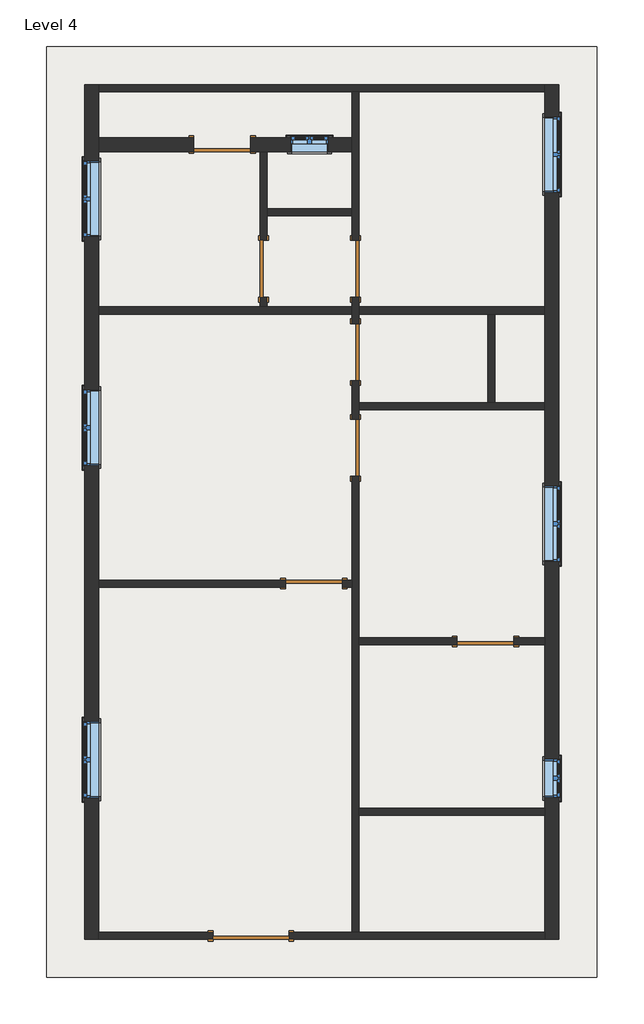
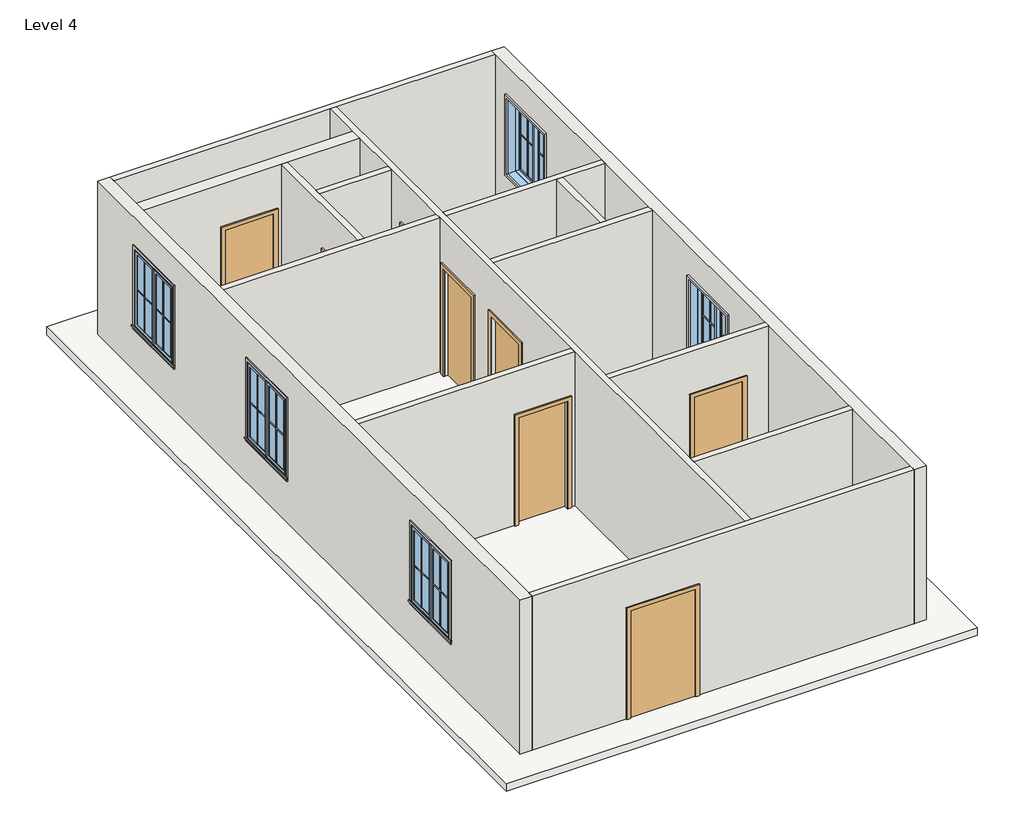
# One storey, incomplete: 28 proxies, 15 walls, 8 doors, 7 windows, 1 slab.
"""IFC4 building model written with IfcOpenShell, lengths in millimetres."""

from ifc_helpers import new_model, si_unit, frame, origin, place, context, project, spatial, polyline, outline, extrude, faceted_brep, transform, mapped, element, save
from components import muntin_pattern_2x2_muntin_pattern_2x2_6dad3731, muntin_pattern_2x2_muntin_pattern_2x2_a30a3345, muntin_pattern_2x2_muntin_pattern_2x2_53152e2c, muntin_pattern_2x2_muntin_pattern_2x2_e8f3e573, trim_window_exterior_flat_with_sill_92b9b949, trim_window_exterior_flat_with_sill_a665a915, trim_window_interior_flat_picture_frame_3bb882cf, trim_window_interior_flat_picture_frame_d485c387, door_a90ba1ad, door_e5f9f3c4, door_305aa2a5, door_6ea84ebe, window_c417fced, window_8377141f

model = new_model("IFC4")

# Units and contexts
model_context = context("Model", 3, world=origin())
ifc_project = project(units=[si_unit("LENGTHUNIT", "METRE", prefix="MILLI")], contexts=[model_context])

# Site, building, storey
site = spatial("IfcSite", under=ifc_project)
building = spatial("IfcBuilding", under=site)
storey = spatial("IfcBuildingStorey", under=building, Name="Level 4", Elevation=9144.0)

# Proxies
placement = place(None, origin())
muntin_pattern_2x2_muntin_pattern_2x2_shape = muntin_pattern_2x2_muntin_pattern_2x2_6dad3731(model_context)
element("IfcBuildingElementProxy", 1, Name="Muntin Pattern_2x2 : Muntin Pattern_2x2", ObjectType="Muntin Pattern_2x2 : Muntin Pattern_2x2", at=placement, inside=storey, context=model_context, shape_type="MappedRepresentation", body=[
    mapped(muntin_pattern_2x2_muntin_pattern_2x2_shape, transform((1279.525, 8669.3375, 10128.25), x_axis=(0.0, 1.0, 0.0), y_axis=(-1.0, 0.0, 0.0), z_axis=(0.0, 0.0, 1.0))),
])
element("IfcBuildingElementProxy", 2, Name="Muntin Pattern_2x2 : Muntin Pattern_2x2", ObjectType="Muntin Pattern_2x2 : Muntin Pattern_2x2", at=placement, inside=storey, context=model_context, shape_type="MappedRepresentation", body=[
    mapped(muntin_pattern_2x2_muntin_pattern_2x2_shape, transform((1279.525, 3341.6875, 10128.25), x_axis=(0.0, 1.0, 0.0), y_axis=(-1.0, 0.0, 0.0), z_axis=(0.0, 0.0, 1.0))),
])
element("IfcBuildingElementProxy", 3, Name="Muntin Pattern_2x2 : Muntin Pattern_2x2", ObjectType="Muntin Pattern_2x2 : Muntin Pattern_2x2", at=placement, inside=storey, context=model_context, shape_type="MappedRepresentation", body=[
    mapped(muntin_pattern_2x2_muntin_pattern_2x2_shape, transform((8880.475, 7732.7125, 10128.25), x_axis=(0.0, -1.0, 0.0), y_axis=(1.0, 0.0, 0.0), z_axis=(0.0, 0.0, 1.0))),
])
element("IfcBuildingElementProxy", 4, Name="Muntin Pattern_2x2 : Muntin Pattern_2x2", ObjectType="Muntin Pattern_2x2 : Muntin Pattern_2x2", at=placement, inside=storey, context=model_context, shape_type="MappedRepresentation", body=[
    mapped(muntin_pattern_2x2_muntin_pattern_2x2_shape, transform((8880.475, 13657.2625, 10128.25), x_axis=(0.0, -1.0, 0.0), y_axis=(1.0, 0.0, 0.0), z_axis=(0.0, 0.0, 1.0))),
])
element("IfcBuildingElementProxy", 5, Name="Muntin Pattern_2x2 : Muntin Pattern_2x2", ObjectType="Muntin Pattern_2x2 : Muntin Pattern_2x2", at=placement, inside=storey, context=model_context, shape_type="MappedRepresentation", body=[
    mapped(muntin_pattern_2x2_muntin_pattern_2x2_shape, transform((1279.525, 12339.6375, 10128.25), x_axis=(0.0, 1.0, 0.0), y_axis=(-1.0, 0.0, 0.0), z_axis=(0.0, 0.0, 1.0))),
])
muntin_pattern_2x2_muntin_pattern_2x2_2_shape = muntin_pattern_2x2_muntin_pattern_2x2_a30a3345(model_context)
element("IfcBuildingElementProxy", 6, Name="Muntin Pattern_2x2 : Muntin Pattern_2x2", ObjectType="Muntin Pattern_2x2 : Muntin Pattern_2x2", at=placement, inside=storey, context=model_context, shape_type="MappedRepresentation", body=[
    mapped(muntin_pattern_2x2_muntin_pattern_2x2_2_shape, transform((1279.525, 9275.7625, 10128.25), x_axis=(0.0, -1.0, 0.0), y_axis=(1.0, 0.0, 0.0), z_axis=(0.0, 0.0, 1.0))),
])
element("IfcBuildingElementProxy", 7, Name="Muntin Pattern_2x2 : Muntin Pattern_2x2", ObjectType="Muntin Pattern_2x2 : Muntin Pattern_2x2", at=placement, inside=storey, context=model_context, shape_type="MappedRepresentation", body=[
    mapped(muntin_pattern_2x2_muntin_pattern_2x2_2_shape, transform((1279.525, 3948.1125, 10128.25), x_axis=(0.0, -1.0, 0.0), y_axis=(1.0, 0.0, 0.0), z_axis=(0.0, 0.0, 1.0))),
])
element("IfcBuildingElementProxy", 8, Name="Muntin Pattern_2x2 : Muntin Pattern_2x2", ObjectType="Muntin Pattern_2x2 : Muntin Pattern_2x2", at=placement, inside=storey, context=model_context, shape_type="MappedRepresentation", body=[
    mapped(muntin_pattern_2x2_muntin_pattern_2x2_2_shape, transform((8880.475, 7126.2875, 10128.25), x_axis=(0.0, 1.0, 0.0), y_axis=(-1.0, 0.0, 0.0), z_axis=(0.0, 0.0, 1.0))),
])
element("IfcBuildingElementProxy", 9, Name="Muntin Pattern_2x2 : Muntin Pattern_2x2", ObjectType="Muntin Pattern_2x2 : Muntin Pattern_2x2", at=placement, inside=storey, context=model_context, shape_type="MappedRepresentation", body=[
    mapped(muntin_pattern_2x2_muntin_pattern_2x2_2_shape, transform((8880.475, 13050.8375, 10128.25), x_axis=(0.0, 1.0, 0.0), y_axis=(-1.0, 0.0, 0.0), z_axis=(0.0, 0.0, 1.0))),
])
element("IfcBuildingElementProxy", 10, Name="Muntin Pattern_2x2 : Muntin Pattern_2x2", ObjectType="Muntin Pattern_2x2 : Muntin Pattern_2x2", at=placement, inside=storey, context=model_context, shape_type="MappedRepresentation", body=[
    mapped(muntin_pattern_2x2_muntin_pattern_2x2_2_shape, transform((1279.525, 12946.0625, 10128.25), x_axis=(0.0, -1.0, 0.0), y_axis=(1.0, 0.0, 0.0), z_axis=(0.0, 0.0, 1.0))),
])
muntin_pattern_2x2_muntin_pattern_2x2_3_shape = muntin_pattern_2x2_muntin_pattern_2x2_53152e2c(model_context)
element("IfcBuildingElementProxy", 11, Name="Muntin Pattern_2x2 : Muntin Pattern_2x2", ObjectType="Muntin Pattern_2x2 : Muntin Pattern_2x2", at=placement, inside=storey, context=model_context, shape_type="MappedRepresentation", body=[
    mapped(muntin_pattern_2x2_muntin_pattern_2x2_3_shape, transform((4732.3375, 13617.575, 10128.25), x_axis=(1.0, 0.0, 0.0), y_axis=(0.0, 1.0, 0.0), z_axis=(0.0, 0.0, 1.0))),
])
element("IfcBuildingElementProxy", 12, Name="Muntin Pattern_2x2 : Muntin Pattern_2x2", ObjectType="Muntin Pattern_2x2 : Muntin Pattern_2x2", at=placement, inside=storey, context=model_context, shape_type="MappedRepresentation", body=[
    mapped(muntin_pattern_2x2_muntin_pattern_2x2_3_shape, transform((8880.475, 3497.2625, 10128.25), x_axis=(0.0, -1.0, 0.0), y_axis=(1.0, 0.0, 0.0), z_axis=(0.0, 0.0, 1.0))),
])
muntin_pattern_2x2_muntin_pattern_2x2_4_shape = muntin_pattern_2x2_muntin_pattern_2x2_e8f3e573(model_context)
element("IfcBuildingElementProxy", 13, Name="Muntin Pattern_2x2 : Muntin Pattern_2x2", ObjectType="Muntin Pattern_2x2 : Muntin Pattern_2x2", at=placement, inside=storey, context=model_context, shape_type="MappedRepresentation", body=[
    mapped(muntin_pattern_2x2_muntin_pattern_2x2_4_shape, transform((5033.9625, 13617.575, 10128.25), x_axis=(-1.0, 0.0, 0.0), y_axis=(0.0, -1.0, 0.0), z_axis=(0.0, 0.0, 1.0))),
])
element("IfcBuildingElementProxy", 14, Name="Muntin Pattern_2x2 : Muntin Pattern_2x2", ObjectType="Muntin Pattern_2x2 : Muntin Pattern_2x2", at=placement, inside=storey, context=model_context, shape_type="MappedRepresentation", body=[
    mapped(muntin_pattern_2x2_muntin_pattern_2x2_4_shape, transform((8880.475, 3195.6375, 10128.25), x_axis=(0.0, 1.0, 0.0), y_axis=(-1.0, 0.0, 0.0), z_axis=(0.0, 0.0, 1.0))),
])
trim_window_exterior_flat_with_sill_shape = trim_window_exterior_flat_with_sill_92b9b949(model_context)
element("IfcBuildingElementProxy", 15, Name="Trim-Window-Exterior-Flat : with Sill", ObjectType="Trim-Window-Exterior-Flat : with Sill", at=placement, inside=storey, context=model_context, shape_type="MappedRepresentation", body=[
    mapped(trim_window_exterior_flat_with_sill_shape, transform((1270.0, 8972.55, 11582.4), x_axis=(0.0, -1.0, 0.0), y_axis=(0.0, 0.0, 1.0), z_axis=(-1.0, 0.0, 0.0))),
])
element("IfcBuildingElementProxy", 16, Name="Trim-Window-Exterior-Flat : with Sill", ObjectType="Trim-Window-Exterior-Flat : with Sill", at=placement, inside=storey, context=model_context, shape_type="MappedRepresentation", body=[
    mapped(trim_window_exterior_flat_with_sill_shape, transform((1270.0, 3644.9, 11582.4), x_axis=(0.0, -1.0, 0.0), y_axis=(0.0, 0.0, 1.0), z_axis=(-1.0, 0.0, 0.0))),
])
element("IfcBuildingElementProxy", 17, Name="Trim-Window-Exterior-Flat : with Sill", ObjectType="Trim-Window-Exterior-Flat : with Sill", at=placement, inside=storey, context=model_context, shape_type="MappedRepresentation", body=[
    mapped(trim_window_exterior_flat_with_sill_shape, transform((8890.0, 7429.5, 11582.4), x_axis=(0.0, 1.0, 0.0), y_axis=(0.0, 0.0, 1.0), z_axis=(1.0, 0.0, 0.0))),
])
element("IfcBuildingElementProxy", 18, Name="Trim-Window-Exterior-Flat : with Sill", ObjectType="Trim-Window-Exterior-Flat : with Sill", at=placement, inside=storey, context=model_context, shape_type="MappedRepresentation", body=[
    mapped(trim_window_exterior_flat_with_sill_shape, transform((8890.0, 13354.05, 11582.4), x_axis=(0.0, 1.0, 0.0), y_axis=(0.0, 0.0, 1.0), z_axis=(1.0, 0.0, 0.0))),
])
element("IfcBuildingElementProxy", 19, Name="Trim-Window-Exterior-Flat : with Sill", ObjectType="Trim-Window-Exterior-Flat : with Sill", at=placement, inside=storey, context=model_context, shape_type="MappedRepresentation", body=[
    mapped(trim_window_exterior_flat_with_sill_shape, transform((1270.0, 12642.85, 11582.4), x_axis=(0.0, -1.0, 0.0), y_axis=(0.0, 0.0, 1.0), z_axis=(-1.0, 0.0, 0.0))),
])
trim_window_exterior_flat_with_sill_2_shape = trim_window_exterior_flat_with_sill_a665a915(model_context)
element("IfcBuildingElementProxy", 20, Name="Trim-Window-Exterior-Flat : with Sill", ObjectType="Trim-Window-Exterior-Flat : with Sill", at=placement, inside=storey, context=model_context, shape_type="MappedRepresentation", body=[
    mapped(trim_window_exterior_flat_with_sill_2_shape, transform((4883.15, 13627.1, 10972.8), x_axis=(-1.0, 0.0, 0.0), y_axis=(0.0, 0.0, 1.0), z_axis=(0.0, 1.0, 0.0))),
])
element("IfcBuildingElementProxy", 21, Name="Trim-Window-Exterior-Flat : with Sill", ObjectType="Trim-Window-Exterior-Flat : with Sill", at=placement, inside=storey, context=model_context, shape_type="MappedRepresentation", body=[
    mapped(trim_window_exterior_flat_with_sill_2_shape, transform((8890.0, 3346.45, 10972.8), x_axis=(0.0, 1.0, 0.0), y_axis=(0.0, 0.0, 1.0), z_axis=(1.0, 0.0, 0.0))),
])
trim_window_interior_flat_picture_frame_shape = trim_window_interior_flat_picture_frame_3bb882cf(model_context)
element("IfcBuildingElementProxy", 22, Name="Trim-Window-Interior-Flat : Picture Frame", ObjectType="Trim-Window-Interior-Flat : Picture Frame", at=placement, inside=storey, context=model_context, shape_type="MappedRepresentation", body=[
    mapped(trim_window_interior_flat_picture_frame_shape, transform((1498.6, 8972.55, 11582.4), x_axis=(0.0, 1.0, 0.0), y_axis=(0.0, 0.0, 1.0), z_axis=(1.0, 0.0, 0.0))),
])
element("IfcBuildingElementProxy", 23, Name="Trim-Window-Interior-Flat : Picture Frame", ObjectType="Trim-Window-Interior-Flat : Picture Frame", at=placement, inside=storey, context=model_context, shape_type="MappedRepresentation", body=[
    mapped(trim_window_interior_flat_picture_frame_shape, transform((1498.6, 3644.9, 11582.4), x_axis=(0.0, 1.0, 0.0), y_axis=(0.0, 0.0, 1.0), z_axis=(1.0, 0.0, 0.0))),
])
element("IfcBuildingElementProxy", 24, Name="Trim-Window-Interior-Flat : Picture Frame", ObjectType="Trim-Window-Interior-Flat : Picture Frame", at=placement, inside=storey, context=model_context, shape_type="MappedRepresentation", body=[
    mapped(trim_window_interior_flat_picture_frame_shape, transform((8661.4, 7429.5, 11582.4), x_axis=(0.0, -1.0, 0.0), y_axis=(0.0, 0.0, 1.0), z_axis=(-1.0, 0.0, 0.0))),
])
element("IfcBuildingElementProxy", 25, Name="Trim-Window-Interior-Flat : Picture Frame", ObjectType="Trim-Window-Interior-Flat : Picture Frame", at=placement, inside=storey, context=model_context, shape_type="MappedRepresentation", body=[
    mapped(trim_window_interior_flat_picture_frame_shape, transform((8661.4, 13354.05, 11582.4), x_axis=(0.0, -1.0, 0.0), y_axis=(0.0, 0.0, 1.0), z_axis=(-1.0, 0.0, 0.0))),
])
element("IfcBuildingElementProxy", 26, Name="Trim-Window-Interior-Flat : Picture Frame", ObjectType="Trim-Window-Interior-Flat : Picture Frame", at=placement, inside=storey, context=model_context, shape_type="MappedRepresentation", body=[
    mapped(trim_window_interior_flat_picture_frame_shape, transform((1498.6, 12642.85, 11582.4), x_axis=(0.0, 1.0, 0.0), y_axis=(0.0, 0.0, 1.0), z_axis=(1.0, 0.0, 0.0))),
])
trim_window_interior_flat_picture_frame_2_shape = trim_window_interior_flat_picture_frame_d485c387(model_context)
element("IfcBuildingElementProxy", 27, Name="Trim-Window-Interior-Flat : Picture Frame", ObjectType="Trim-Window-Interior-Flat : Picture Frame", at=placement, inside=storey, context=model_context, shape_type="MappedRepresentation", body=[
    mapped(trim_window_interior_flat_picture_frame_2_shape, transform((4883.15, 13398.5, 10972.8), x_axis=(1.0, 0.0, 0.0), y_axis=(0.0, 0.0, 1.0), z_axis=(0.0, -1.0, 0.0))),
])
element("IfcBuildingElementProxy", 28, Name="Trim-Window-Interior-Flat : Picture Frame", ObjectType="Trim-Window-Interior-Flat : Picture Frame", at=placement, inside=storey, context=model_context, shape_type="MappedRepresentation", body=[
    mapped(trim_window_interior_flat_picture_frame_2_shape, transform((8661.4, 3346.45, 10972.8), x_axis=(0.0, -1.0, 0.0), y_axis=(0.0, 0.0, 1.0), z_axis=(-1.0, 0.0, 0.0))),
])

# Doors
door_shape = door_a90ba1ad(model_context)
element("IfcDoor", 29, ObjectType="Single-Flush : 36\" x 84\"", at=placement, inside=storey, context=model_context, shape_type="MappedRepresentation", body=[
    mapped(door_shape, transform((3479.8, 13512.8, 9144.0), x_axis=(1.0, 0.0, 0.0), y_axis=(0.0, 1.0, 0.0), z_axis=(0.0, 0.0, 1.0))),
])
door_2_shape = door_e5f9f3c4(model_context)
element("IfcDoor", 30, ObjectType="Single-Flush : 36\" x 84\"", at=placement, inside=storey, context=model_context, shape_type="MappedRepresentation", body=[
    mapped(door_2_shape, transform((5619.75, 11518.9, 9144.0), x_axis=(0.0, -1.0, 0.0), y_axis=(1.0, 0.0, 0.0), z_axis=(0.0, 0.0, 1.0))),
])
element("IfcDoor", 31, ObjectType="Single-Flush : 36\" x 84\"", at=placement, inside=storey, context=model_context, shape_type="MappedRepresentation", body=[
    mapped(door_2_shape, transform((4953.0, 6470.65, 9144.0), x_axis=(1.0, 0.0, 0.0), y_axis=(0.0, 1.0, 0.0), z_axis=(0.0, 0.0, 1.0))),
])
element("IfcDoor", 32, ObjectType="Single-Flush : 36\" x 84\"", at=placement, inside=storey, context=model_context, shape_type="MappedRepresentation", body=[
    mapped(door_2_shape, transform((7708.9, 5543.55, 9144.0), x_axis=(-1.0, 0.0, 0.0), y_axis=(0.0, -1.0, 0.0), z_axis=(0.0, 0.0, 1.0))),
])
door_3_shape = door_305aa2a5(model_context)
element("IfcDoor", 33, ObjectType="Single-Flush : 36\" x 84\"", at=placement, inside=storey, context=model_context, shape_type="MappedRepresentation", body=[
    mapped(door_3_shape, transform((4146.55, 11518.9, 9144.0), x_axis=(0.0, -1.0, 0.0), y_axis=(1.0, 0.0, 0.0), z_axis=(0.0, 0.0, 1.0))),
])
element("IfcDoor", 34, ObjectType="Single-Flush : 36\" x 84\"", at=placement, inside=storey, context=model_context, shape_type="MappedRepresentation", body=[
    mapped(door_3_shape, transform((5619.75, 10185.4, 9144.0), x_axis=(0.0, 1.0, 0.0), y_axis=(-1.0, 0.0, 0.0), z_axis=(0.0, 0.0, 1.0))),
])
element("IfcDoor", 35, ObjectType="Single-Flush : 36\" x 84\"", at=placement, inside=storey, context=model_context, shape_type="MappedRepresentation", body=[
    mapped(door_3_shape, transform((5619.75, 8648.7, 9144.0), x_axis=(0.0, 1.0, 0.0), y_axis=(-1.0, 0.0, 0.0), z_axis=(0.0, 0.0, 1.0))),
])
door_4_shape = door_6ea84ebe(model_context)
element("IfcDoor", 36, ObjectType="Single-Flush : 48\" x 84\"", at=placement, inside=storey, context=model_context, shape_type="MappedRepresentation", body=[
    mapped(door_4_shape, transform((3943.35, 819.15, 9144.0), x_axis=(-1.0, 0.0, 0.0), y_axis=(0.0, -1.0, 0.0), z_axis=(0.0, 0.0, 1.0))),
])

# Slab
element("IfcSlab", 37, ObjectType="Generic - 12\"", at=placement, inside=storey, context=model_context, shape_type="SweptSolid", body=[
    extrude(outline(polyline([(9499.6, 15087.6), (9499.6, 152.4), (660.4, 152.4), (660.4, 15087.6), (9499.6, 15087.6)])), frame((0.0, 0.0, 8991.6), z_axis=(0.0, 0.0, 1.0), x_axis=(1.0, 0.0, 0.0)), (0.0, 0.0, 1.0), 152.4),
])

# Walls
element("IfcWall", 38, ObjectType="Generic - 5\"", at=placement, inside=storey, context=model_context, shape_type="Brep", body=[
    faceted_brep([(1498.6, 14363.7, 9144.0), (5562.6, 14363.7, 9144.0), (5676.9, 14363.7, 9144.0), (8661.4, 14363.7, 9144.0), (8661.4, 14363.7, 12192.0), (5676.9, 14363.7, 12192.0), (5562.6, 14363.7, 12192.0), (1498.6, 14363.7, 12192.0), (1498.6, 14478.0, 9144.0), (1498.6, 14478.0, 12192.0), (8661.4, 14478.0, 12192.0), (8661.4, 14478.0, 9144.0)], [[[0, 1, 2, 3, 4, 5, 6, 7]], [[8, 9, 10, 11]], [[3, 2, 1, 0, 8, 11]], [[7, 6, 5, 4, 10, 9]], [[4, 3, 11, 10]], [[0, 7, 9, 8]]]),
])
element("IfcWall", 39, ObjectType="Generic - 5\"", at=placement, inside=storey, context=model_context, shape_type="Brep", body=[
    faceted_brep([(1498.6, 762.0, 9144.0), (3333.75, 762.0, 9144.0), (3333.75, 762.0, 11277.6), (4552.95, 762.0, 11277.6), (4552.95, 762.0, 9144.0), (8661.4, 762.0, 9144.0), (8661.4, 762.0, 12192.0), (1498.6, 762.0, 12192.0), (3333.75, 876.3, 11277.6), (3333.75, 876.3, 9144.0), (1498.6, 876.3, 9144.0), (1498.6, 876.3, 12192.0), (5562.6, 876.3, 12192.0), (5676.9, 876.3, 12192.0), (8661.4, 876.3, 12192.0), (8661.4, 876.3, 9144.0), (5676.9, 876.3, 9144.0), (5562.6, 876.3, 9144.0), (4552.95, 876.3, 9144.0), (4552.95, 876.3, 11277.6)], [[[0, 1, 2, 3, 4, 5, 6, 7]], [[8, 9, 10, 11, 12, 13, 14, 15, 16, 17, 18, 19]], [[10, 9, 1, 0]], [[18, 17, 16, 15, 5, 4]], [[7, 6, 14, 13, 12, 11]], [[6, 5, 15, 14]], [[0, 7, 11, 10]], [[2, 1, 9, 8]], [[3, 2, 8, 19]], [[4, 3, 19, 18]]]),
])
element("IfcWall", 40, ObjectType="Generic - 5\"", at=placement, inside=storey, context=model_context, shape_type="Brep", body=[
    faceted_brep([(5562.6, 9728.2, 9144.0), (5562.6, 9105.9, 9144.0), (5562.6, 9105.9, 11277.6), (5562.6, 8191.5, 11277.6), (5562.6, 8191.5, 9144.0), (5562.6, 6527.8, 9144.0), (5562.6, 6413.5, 9144.0), (5562.6, 876.3, 9144.0), (5562.6, 876.3, 12192.0), (5562.6, 6413.5, 12192.0), (5562.6, 6527.8, 12192.0), (5562.6, 10795.0, 12192.0), (5562.6, 10909.3, 12192.0), (5562.6, 12369.8, 12192.0), (5562.6, 12484.1, 12192.0), (5562.6, 13398.5, 12192.0), (5562.6, 13627.1, 12192.0), (5562.6, 14363.7, 12192.0), (5562.6, 14363.7, 9144.0), (5562.6, 13627.1, 9144.0), (5562.6, 13398.5, 9144.0), (5562.6, 12484.1, 9144.0), (5562.6, 12369.8, 9144.0), (5562.6, 11976.1, 9144.0), (5562.6, 11976.1, 11277.6), (5562.6, 11061.7, 11277.6), (5562.6, 11061.7, 9144.0), (5562.6, 10909.3, 9144.0), (5562.6, 10795.0, 9144.0), (5562.6, 10642.6, 9144.0), (5562.6, 10642.6, 11277.6), (5562.6, 9728.2, 11277.6), (5676.9, 9105.9, 11277.6), (5676.9, 9105.9, 9144.0), (5676.9, 9258.3, 9144.0), (5676.9, 9372.6, 9144.0), (5676.9, 9728.2, 9144.0), (5676.9, 9728.2, 11277.6), (5676.9, 10642.6, 11277.6), (5676.9, 10642.6, 9144.0), (5676.9, 10795.0, 9144.0), (5676.9, 10909.3, 9144.0), (5676.9, 11061.7, 9144.0), (5676.9, 11061.7, 11277.6), (5676.9, 11976.1, 11277.6), (5676.9, 11976.1, 9144.0), (5676.9, 14363.7, 9144.0), (5676.9, 14363.7, 12192.0), (5676.9, 10909.3, 12192.0), (5676.9, 10795.0, 12192.0), (5676.9, 9372.6, 12192.0), (5676.9, 9258.3, 12192.0), (5676.9, 5600.7, 12192.0), (5676.9, 5486.4, 12192.0), (5676.9, 2870.2, 12192.0), (5676.9, 2755.9, 12192.0), (5676.9, 876.3, 12192.0), (5676.9, 876.3, 9144.0), (5676.9, 2755.9, 9144.0), (5676.9, 2870.2, 9144.0), (5676.9, 5486.4, 9144.0), (5676.9, 5600.7, 9144.0), (5676.9, 8191.5, 9144.0), (5676.9, 8191.5, 11277.6)], [[[0, 1, 2, 3, 4, 5, 6, 7, 8, 9, 10, 11, 12, 13, 14, 15, 16, 17, 18, 19, 20, 21, 22, 23, 24, 25, 26, 27, 28, 29, 30, 31]], [[32, 33, 34, 35, 36, 37, 38, 39, 40, 41, 42, 43, 44, 45, 46, 47, 48, 49, 50, 51, 52, 53, 54, 55, 56, 57, 58, 59, 60, 61, 62, 63]], [[23, 22, 21, 20, 19, 18, 46, 45]], [[42, 41, 40, 39, 29, 28, 27, 26]], [[36, 35, 34, 33, 1, 0]], [[62, 61, 60, 59, 58, 57, 7, 6, 5, 4]], [[17, 16, 15, 14, 13, 12, 11, 10, 9, 8, 56, 55, 54, 53, 52, 51, 50, 49, 48, 47]], [[18, 17, 47, 46]], [[8, 7, 57, 56]], [[43, 42, 26, 25]], [[44, 43, 25, 24]], [[45, 44, 24, 23]], [[30, 29, 39, 38]], [[31, 30, 38, 37]], [[0, 31, 37, 36]], [[2, 1, 33, 32]], [[3, 2, 32, 63]], [[4, 3, 63, 62]]]),
])
element("IfcWall", 41, ObjectType="Generic - 5\"", at=placement, inside=storey, context=model_context, shape_type="SweptSolid", body=[
    extrude(outline(polyline([(9144.0, 5676.9), (9144.0, 7251.7), (11277.6, 7251.7), (11277.6, 8166.1), (9144.0, 8166.1), (9144.0, 8661.4), (12192.0, 8661.4), (12192.0, 5676.9), (9144.0, 5676.9)])), frame((0.0, 5486.4, 0.0), z_axis=(0.0, 1.0, 0.0), x_axis=(0.0, 0.0, 1.0)), (0.0, 0.0, 1.0), 114.3),
])
element("IfcWall", 42, ObjectType="Generic - 5\"", at=placement, inside=storey, context=model_context, shape_type="SweptSolid", body=[
    extrude(outline(polyline([(11277.6, 5410.2), (9144.0, 5410.2), (9144.0, 5562.6), (12192.0, 5562.6), (12192.0, 1498.6), (9144.0, 1498.6), (9144.0, 4495.8), (11277.6, 4495.8), (11277.6, 5410.2)])), frame((0.0, 6413.5, 0.0), z_axis=(0.0, 1.0, 0.0), x_axis=(0.0, 0.0, 1.0)), (0.0, 0.0, 1.0), 114.3),
])
element("IfcWall", 43, ObjectType="Generic - 5\"", at=placement, inside=storey, context=model_context, shape_type="Brep", body=[
    faceted_brep([(1498.6, 10795.0, 9144.0), (5562.6, 10795.0, 9144.0), (5562.6, 10795.0, 12192.0), (1498.6, 10795.0, 12192.0), (1498.6, 10909.3, 9144.0), (1498.6, 10909.3, 12192.0), (4089.4, 10909.3, 12192.0), (4203.7, 10909.3, 12192.0), (5562.6, 10909.3, 12192.0), (5562.6, 10909.3, 9144.0), (4203.7, 10909.3, 9144.0), (4089.4, 10909.3, 9144.0)], [[[0, 1, 2, 3]], [[4, 5, 6, 7, 8, 9, 10, 11]], [[1, 0, 4, 11, 10, 9]], [[3, 2, 8, 7, 6, 5]], [[0, 3, 5, 4]], [[2, 1, 9, 8]]]),
])
element("IfcWall", 44, ObjectType="Generic - 5\"", at=placement, inside=storey, context=model_context, shape_type="Brep", body=[
    faceted_brep([(5676.9, 10795.0, 9144.0), (7747.0010433, 10795.0, 9144.0), (7861.3010433, 10795.0, 9144.0), (8661.4, 10795.0, 9144.0), (8661.4, 10795.0, 12192.0), (7861.3010433, 10795.0, 12192.0), (7747.0010433, 10795.0, 12192.0), (5676.9, 10795.0, 12192.0), (5676.9, 10909.3, 9144.0), (5676.9, 10909.3, 12192.0), (8661.4, 10909.3, 12192.0), (8661.4, 10909.3, 9144.0)], [[[0, 1, 2, 3, 4, 5, 6, 7]], [[8, 9, 10, 11]], [[3, 2, 1, 0, 8, 11]], [[7, 6, 5, 4, 10, 9]], [[4, 3, 11, 10]], [[0, 7, 9, 8]]]),
])
element("IfcWall", 45, ObjectType="Generic - 5\"", at=placement, inside=storey, context=model_context, shape_type="SweptSolid", body=[
    extrude(outline(polyline([(7747.0010433, 9372.6), (7747.0010433, 10795.0), (7861.3010433, 10795.0), (7861.3010433, 9372.6), (7747.0010433, 9372.6)])), frame((0.0, 0.0, 9144.0), z_axis=(0.0, 0.0, 1.0), x_axis=(1.0, 0.0, 0.0)), (0.0, 0.0, 1.0), 3048.0),
])
element("IfcWall", 46, ObjectType="Generic - 5\"", at=placement, inside=storey, context=model_context, shape_type="Brep", body=[
    faceted_brep([(5676.9, 9258.3, 9144.0), (8661.4, 9258.3, 9144.0), (8661.4, 9258.3, 12192.0), (5676.9, 9258.3, 12192.0), (5676.9, 9372.6, 9144.0), (5676.9, 9372.6, 12192.0), (7747.0010433, 9372.6, 12192.0), (7861.3010433, 9372.6, 12192.0), (8661.4, 9372.6, 12192.0), (8661.4, 9372.6, 9144.0), (7861.3010433, 9372.6, 9144.0), (7747.0010433, 9372.6, 9144.0)], [[[0, 1, 2, 3]], [[4, 5, 6, 7, 8, 9, 10, 11]], [[1, 0, 4, 11, 10, 9]], [[3, 2, 8, 7, 6, 5]], [[2, 1, 9, 8]], [[0, 3, 5, 4]]]),
])
element("IfcWall", 47, ObjectType="Generic - 5\"", at=placement, inside=storey, context=model_context, shape_type="SweptSolid", body=[
    extrude(outline(polyline([(8661.4, 2755.9), (5676.9, 2755.9), (5676.9, 2870.2), (8661.4, 2870.2), (8661.4, 2755.9)])), frame((0.0, 0.0, 9144.0), z_axis=(0.0, 0.0, 1.0), x_axis=(1.0, 0.0, 0.0)), (0.0, 0.0, 1.0), 3048.0),
])
element("IfcWall", 48, ObjectType="Generic - 5\"", at=placement, inside=storey, context=model_context, shape_type="Brep", body=[
    faceted_brep([(4203.7, 10909.3, 9144.0), (4203.7, 11061.7, 9144.0), (4203.7, 11061.7, 11277.6), (4203.7, 11976.1, 11277.6), (4203.7, 11976.1, 9144.0), (4203.7, 12369.8, 9144.0), (4203.7, 12484.1, 9144.0), (4203.7, 13398.5, 9144.0), (4203.7, 13398.5, 12192.0), (4203.7, 12484.1, 12192.0), (4203.7, 12369.8, 12192.0), (4203.7, 10909.3, 12192.0), (4089.4, 11061.7, 11277.6), (4089.4, 11061.7, 9144.0), (4089.4, 10909.3, 9144.0), (4089.4, 10909.3, 12192.0), (4089.4, 13398.5, 12192.0), (4089.4, 13398.5, 9144.0), (4089.4, 11976.1, 9144.0), (4089.4, 11976.1, 11277.6)], [[[0, 1, 2, 3, 4, 5, 6, 7, 8, 9, 10, 11]], [[12, 13, 14, 15, 16, 17, 18, 19]], [[18, 17, 7, 6, 5, 4]], [[14, 13, 1, 0]], [[11, 10, 9, 8, 16, 15]], [[0, 11, 15, 14]], [[8, 7, 17, 16]], [[2, 1, 13, 12]], [[3, 2, 12, 19]], [[4, 3, 19, 18]]]),
])
element("IfcWall", 49, ObjectType="Generic - 5\"", at=placement, inside=storey, context=model_context, shape_type="SweptSolid", body=[
    extrude(outline(polyline([(5562.6, 12369.8), (4203.7, 12369.8), (4203.7, 12484.1), (5562.6, 12484.1), (5562.6, 12369.8)])), frame((0.0, 0.0, 9144.0), z_axis=(0.0, 0.0, 1.0), x_axis=(1.0, 0.0, 0.0)), (0.0, 0.0, 1.0), 3048.0),
])
element("IfcWall", 50, ObjectType="Generic - 8\"", at=placement, inside=storey, context=model_context, shape_type="Brep", body=[
    faceted_brep([(8661.4, 14478.0, 9144.0), (8661.4, 14363.7, 9144.0), (8661.4, 10909.3, 9144.0), (8661.4, 10795.0, 9144.0), (8661.4, 9372.6, 9144.0), (8661.4, 9258.3, 9144.0), (8661.4, 5600.7, 9144.0), (8661.4, 5486.4, 9144.0), (8661.4, 2870.2, 9144.0), (8661.4, 2755.9, 9144.0), (8661.4, 876.3, 9144.0), (8661.4, 762.0, 9144.0), (8661.4, 762.0, 12192.0), (8661.4, 876.3, 12192.0), (8661.4, 2755.9, 12192.0), (8661.4, 2870.2, 12192.0), (8661.4, 5486.4, 12192.0), (8661.4, 5600.7, 12192.0), (8661.4, 9258.3, 12192.0), (8661.4, 9372.6, 12192.0), (8661.4, 10795.0, 12192.0), (8661.4, 10909.3, 12192.0), (8661.4, 14363.7, 12192.0), (8661.4, 14478.0, 12192.0), (8661.4, 6819.9, 11582.4), (8661.4, 6819.9, 10058.4), (8661.4, 8039.1, 10058.4), (8661.4, 8039.1, 11582.4), (8661.4, 12744.45, 11582.4), (8661.4, 12744.45, 10058.4), (8661.4, 13963.65, 10058.4), (8661.4, 13963.65, 11582.4), (8661.4, 3041.65, 10972.8), (8661.4, 3041.65, 10058.4), (8661.4, 3651.25, 10058.4), (8661.4, 3651.25, 10972.8), (8890.0, 14478.0, 9144.0), (8890.0, 14478.0, 12192.0), (8890.0, 762.0, 12192.0), (8890.0, 762.0, 9144.0), (8890.0, 6819.9, 11582.4), (8890.0, 8039.1, 11582.4), (8890.0, 8039.1, 10058.4), (8890.0, 6819.9, 10058.4), (8890.0, 12744.45, 11582.4), (8890.0, 13963.65, 11582.4), (8890.0, 13963.65, 10058.4), (8890.0, 12744.45, 10058.4), (8890.0, 3041.65, 10972.8), (8890.0, 3651.25, 10972.8), (8890.0, 3651.25, 10058.4), (8890.0, 3041.65, 10058.4)], [[[0, 1, 2, 3, 4, 5, 6, 7, 8, 9, 10, 11, 12, 13, 14, 15, 16, 17, 18, 19, 20, 21, 22, 23], [24, 25, 26, 27], [28, 29, 30, 31], [32, 33, 34, 35]], [[36, 37, 38, 39], [40, 41, 42, 43], [44, 45, 46, 47], [48, 49, 50, 51]], [[11, 10, 9, 8, 7, 6, 5, 4, 3, 2, 1, 0, 36, 39]], [[23, 22, 21, 20, 19, 18, 17, 16, 15, 14, 13, 12, 38, 37]], [[0, 23, 37, 36]], [[12, 11, 39, 38]], [[25, 24, 40, 43]], [[26, 25, 43, 42]], [[27, 26, 42, 41]], [[24, 27, 41, 40]], [[29, 28, 44, 47]], [[30, 29, 47, 46]], [[31, 30, 46, 45]], [[28, 31, 45, 44]], [[33, 32, 48, 51]], [[34, 33, 51, 50]], [[35, 34, 50, 49]], [[32, 35, 49, 48]]]),
])
element("IfcWall", 51, ObjectType="Generic - 8\"", at=placement, inside=storey, context=model_context, shape_type="Brep", body=[
    faceted_brep([(1270.0, 14478.0, 9144.0), (1270.0, 762.0, 9144.0), (1270.0, 762.0, 12192.0), (1270.0, 14478.0, 12192.0), (1270.0, 9582.15, 11582.4), (1270.0, 8362.95, 11582.4), (1270.0, 8362.95, 10058.4), (1270.0, 9582.15, 10058.4), (1270.0, 4254.5, 11582.4), (1270.0, 3035.3, 11582.4), (1270.0, 3035.3, 10058.4), (1270.0, 4254.5, 10058.4), (1270.0, 13252.45, 11582.4), (1270.0, 12033.25, 11582.4), (1270.0, 12033.25, 10058.4), (1270.0, 13252.45, 10058.4), (1498.6, 14478.0, 9144.0), (1498.6, 14478.0, 12192.0), (1498.6, 14363.7, 12192.0), (1498.6, 13627.1, 12192.0), (1498.6, 13398.5, 12192.0), (1498.6, 10909.3, 12192.0), (1498.6, 10795.0, 12192.0), (1498.6, 6527.8, 12192.0), (1498.6, 6413.5, 12192.0), (1498.6, 876.3, 12192.0), (1498.6, 762.0, 12192.0), (1498.6, 762.0, 9144.0), (1498.6, 876.3, 9144.0), (1498.6, 6413.5, 9144.0), (1498.6, 6527.8, 9144.0), (1498.6, 10795.0, 9144.0), (1498.6, 10909.3, 9144.0), (1498.6, 13398.5, 9144.0), (1498.6, 13627.1, 9144.0), (1498.6, 14363.7, 9144.0), (1498.6, 9582.15, 11582.4), (1498.6, 9582.15, 10058.4), (1498.6, 8362.95, 10058.4), (1498.6, 8362.95, 11582.4), (1498.6, 4254.5, 11582.4), (1498.6, 4254.5, 10058.4), (1498.6, 3035.3, 10058.4), (1498.6, 3035.3, 11582.4), (1498.6, 13252.45, 11582.4), (1498.6, 13252.45, 10058.4), (1498.6, 12033.25, 10058.4), (1498.6, 12033.25, 11582.4)], [[[0, 1, 2, 3], [4, 5, 6, 7], [8, 9, 10, 11], [12, 13, 14, 15]], [[16, 17, 18, 19, 20, 21, 22, 23, 24, 25, 26, 27, 28, 29, 30, 31, 32, 33, 34, 35], [36, 37, 38, 39], [40, 41, 42, 43], [44, 45, 46, 47]], [[1, 0, 16, 35, 34, 33, 32, 31, 30, 29, 28, 27]], [[3, 2, 26, 25, 24, 23, 22, 21, 20, 19, 18, 17]], [[0, 3, 17, 16]], [[2, 1, 27, 26]], [[37, 36, 4, 7]], [[38, 37, 7, 6]], [[39, 38, 6, 5]], [[36, 39, 5, 4]], [[41, 40, 8, 11]], [[42, 41, 11, 10]], [[43, 42, 10, 9]], [[40, 43, 9, 8]], [[45, 44, 12, 15]], [[46, 45, 15, 14]], [[47, 46, 14, 13]], [[44, 47, 13, 12]]]),
])
element("IfcWall", 52, ObjectType="Generic - 8\"", at=placement, inside=storey, context=model_context, shape_type="Brep", body=[
    faceted_brep([(3937.0, 13398.5, 11277.6), (3937.0, 13398.5, 9144.0), (4089.4, 13398.5, 9144.0), (4203.7, 13398.5, 9144.0), (5562.6, 13398.5, 9144.0), (5562.6, 13398.5, 12192.0), (4203.7, 13398.5, 12192.0), (4089.4, 13398.5, 12192.0), (1498.6, 13398.5, 12192.0), (1498.6, 13398.5, 9144.0), (3022.6, 13398.5, 9144.0), (3022.6, 13398.5, 11277.6), (5187.95, 13398.5, 10972.8), (5187.95, 13398.5, 10058.4), (4578.35, 13398.5, 10058.4), (4578.35, 13398.5, 10972.8), (5562.6, 13627.1, 9144.0), (3937.0, 13627.1, 9144.0), (3937.0, 13627.1, 11277.6), (3022.6, 13627.1, 11277.6), (3022.6, 13627.1, 9144.0), (1498.6, 13627.1, 9144.0), (1498.6, 13627.1, 12192.0), (5562.6, 13627.1, 12192.0), (5187.95, 13627.1, 10972.8), (4578.35, 13627.1, 10972.8), (4578.35, 13627.1, 10058.4), (5187.95, 13627.1, 10058.4)], [[[0, 1, 2, 3, 4, 5, 6, 7, 8, 9, 10, 11], [12, 13, 14, 15]], [[16, 17, 18, 19, 20, 21, 22, 23], [24, 25, 26, 27]], [[10, 9, 21, 20]], [[4, 3, 2, 1, 17, 16]], [[8, 7, 6, 5, 23, 22]], [[9, 8, 22, 21]], [[5, 4, 16, 23]], [[18, 17, 1, 0]], [[19, 18, 0, 11]], [[20, 19, 11, 10]], [[13, 12, 24, 27]], [[14, 13, 27, 26]], [[15, 14, 26, 25]], [[12, 15, 25, 24]]]),
])

# Windows
window_shape = window_c417fced(model_context)
element("IfcWindow", 53, ObjectType="Window-Casement-Double : 24\" x 36\"", at=placement, inside=storey, context=model_context, shape_type="MappedRepresentation", body=[
    mapped(window_shape, transform((4883.15, 13512.8, 9144.0), x_axis=(1.0, 0.0, 0.0), y_axis=(0.0, 1.0, 0.0), z_axis=(0.0, 0.0, 1.0))),
])
element("IfcWindow", 54, ObjectType="Window-Casement-Double : 24\" x 36\"", at=placement, inside=storey, context=model_context, shape_type="MappedRepresentation", body=[
    mapped(window_shape, transform((8775.7, 3346.45, 9144.0), x_axis=(0.0, -1.0, 0.0), y_axis=(1.0, 0.0, 0.0), z_axis=(0.0, 0.0, 1.0))),
])
window_2_shape = window_8377141f(model_context)
element("IfcWindow", 55, ObjectType="Window-Casement-Double : 48\" x 60\"", at=placement, inside=storey, context=model_context, shape_type="MappedRepresentation", body=[
    mapped(window_2_shape, transform((1384.3, 8972.55, 9144.0), x_axis=(0.0, 1.0, 0.0), y_axis=(-1.0, 0.0, 0.0), z_axis=(0.0, 0.0, 1.0))),
])
element("IfcWindow", 56, ObjectType="Window-Casement-Double : 48\" x 60\"", at=placement, inside=storey, context=model_context, shape_type="MappedRepresentation", body=[
    mapped(window_2_shape, transform((1384.3, 3644.9, 9144.0), x_axis=(0.0, 1.0, 0.0), y_axis=(-1.0, 0.0, 0.0), z_axis=(0.0, 0.0, 1.0))),
])
element("IfcWindow", 57, ObjectType="Window-Casement-Double : 48\" x 60\"", at=placement, inside=storey, context=model_context, shape_type="MappedRepresentation", body=[
    mapped(window_2_shape, transform((8775.7, 7429.5, 9144.0), x_axis=(0.0, -1.0, 0.0), y_axis=(1.0, 0.0, 0.0), z_axis=(0.0, 0.0, 1.0))),
])
element("IfcWindow", 58, ObjectType="Window-Casement-Double : 48\" x 60\"", at=placement, inside=storey, context=model_context, shape_type="MappedRepresentation", body=[
    mapped(window_2_shape, transform((8775.7, 13354.05, 9144.0), x_axis=(0.0, -1.0, 0.0), y_axis=(1.0, 0.0, 0.0), z_axis=(0.0, 0.0, 1.0))),
])
element("IfcWindow", 59, ObjectType="Window-Casement-Double : 48\" x 60\"", at=placement, inside=storey, context=model_context, shape_type="MappedRepresentation", body=[
    mapped(window_2_shape, transform((1384.3, 12642.85, 9144.0), x_axis=(0.0, 1.0, 0.0), y_axis=(-1.0, 0.0, 0.0), z_axis=(0.0, 0.0, 1.0))),
])

save(model, "model.ifc")

# Revit data of these elements
# Type "Muntin Pattern_2x2 : Muntin Pattern_2x2"
#   Width [instance default] = 4' - 0"
#   Thickness = 0' - 0 1/2"
#   Height [instance default] = 4' - 0"
#   Distance = 0' - 0 3/4"
#   Interior Material [instance default] = none
#   Exterior Material [instance default] = none
#   Default Elevation = 0
# Type "Trim-Window-Exterior-Flat : with Sill"
#   Trim Width = 0' - 2 1/4"
#   Trim Thickness_Picture Frame = 0' - 1 1/4"
#   Trim Thickness_with Sill = 0' - 0 3/4"
#   Sill Thickness = 0' - 1 1/4"
#   Opening Width [instance default] = 2' - 0"
#   Opening Height [instance default] = 3' - 0"
#   Default Elevation = 4' - 0"
#   Sill = yes
#   Picture Frame = no
#   Trim Material [instance default] = none
# Type "Trim-Window-Interior-Flat : Picture Frame"
#   Trim Thickness_Picture Frame = 0' - 1 1/4"
#   Trim Width = 0' - 2 1/4"
#   Trim Thickness_with Sill = 0' - 0 3/4"
#   Sill Thickness = 0' - 1 1/4"
#   Opening Width [instance default] = 2' - 0"
#   Opening Height [instance default] = 3' - 0"
#   Default Elevation = 4' - 0"
#   Sill = no
#   Picture Frame = yes
#   Trim Material [instance default] = none
# Type "Single-Flush : 36\" x 84\""
#   Type Mark = "1"
#   Construction Type Id = "MDOOR"
#   Assembly Code = "C1020"
#   Analytic Construction = "Metal"
#   Thickness = 0' - 2"
#   Heat Transfer Coefficient (U) = 0.651978 BTU/(h·ft²·°F)
#   Height = 7' - 0"
#   Trim Projection Ext = 0' - 1"
#   Trim Projection Int = 0' - 1"
#   Trim Width = 0' - 3"
#   Width = 3' - 0"
#   Define Thermal Properties by = 1
#   Define Thermal Properties by = 1
#   Door Material = Door - Panel
#   Frame Material = Door - Frame
#   Visual Light Transmittance = 0
#   Solar Heat Gain Coefficient = 0
#   Function = (empty or 0)
#   Wall Closure = (empty or 0)
# Type "Single-Flush : 48\" x 84\""
#   Type Mark = "5"
#   Construction Type Id = "MDOOR"
#   Assembly Code = "C1020"
#   Analytic Construction = "Metal"
#   Thickness = 0' - 2"
#   Heat Transfer Coefficient (U) = 0.651978 BTU/(h·ft²·°F)
#   Height = 7' - 0"
#   Trim Projection Ext = 0' - 1"
#   Trim Projection Int = 0' - 1"
#   Trim Width = 0' - 3"
#   Width = 4' - 0"
#   Define Thermal Properties by = 1
#   Define Thermal Properties by = 1
#   Door Material = Door - Panel
#   Frame Material = Door - Frame
#   Visual Light Transmittance = 0
#   Solar Heat Gain Coefficient = 0
#   Function = (empty or 0)
#   Wall Closure = (empty or 0)
# Type "Generic - 12\""
#   Assembly Code = "B1010"
#   Function = 0
#   Layers, outside or top first: 0' - 6" no material (function 1)
# Type "Generic - 5\""
#   Assembly Code = "B2010"
#   Layers, outside or top first: 0' - 4 1/2" no material (function 1)
# Type "Generic - 8\""
#   Assembly Code = "B2010"
#   Layers, outside or top first: 0' - 9" no material (function 1)
# Type "Window-Casement-Double : 24\" x 36\""
#   Type Mark = "14"
#   Fire Rating = "0.5h"
#   Assembly Code = "B2020100"
#   Analytic Construction = "Double glazing - domestic"
#   Frame Extension [instance default] = 0' - 0 1/4"
#   Window Inset [instance default] = 0' - 0"
#   Wall Thickness [instance default] = 0' - 6"
#   Interior Wall Closure [instance default] = 0' - 2 1/4"
#   Half Width = 1' - 0"
#   Visual Light Transmittance = 0.81
#   Thermal Resistance (R) = 1.8146 (h·ft²·°F)/BTU
#   Solar Heat Gain Coefficient = 0.76
#   Rough Width = 2' - 0 1/2"
#   Rough Height = 3' - 0 1/2"
#   Height = 3' - 0"
#   Heat Transfer Coefficient (U) = 0.5511 BTU/(h·ft²·°F)
#   Exterior Wall Closure [instance default] = 0' - 1 1/4"
#   Extension Jamb [instance default] = 0' - 2 1/4"
#   Default Sill Height = 3' - 0"
#   Width = 2' - 0"
#   Define Thermal Properties by = 0
#   Muntin Visibility = yes
#   Interior Trim Visibility [instance default] = yes
#   Exterior Trim Visibility [instance default] = yes
#   Extension Jamb Visibility [instance default] = yes
#   Interior Trim Material = Wood - Stained
#   Muntin Pattern = Muntin Pattern_2x2 : Muntin Pattern_2x2
#   Interior Trim = Trim-Window-Interior-Flat : Picture Frame
#   Interior Frame Material = Wood - Stained
#   Glass Panel Material = Glass
#   Exterior Trim Material = Clad - White
#   Exterior Trim = Trim-Window-Exterior-Flat : with Sill
#   Exterior Frame Material = Clad - White
#   Wall Closure = (empty or 0)
# Type "Window-Casement-Double : 48\" x 60\""
#   Type Mark = "17"
#   Fire Rating = "0.5h"
#   Assembly Code = "B2020100"
#   Analytic Construction = "Double glazing - domestic"
#   Frame Extension [instance default] = 0' - 0 1/4"
#   Window Inset [instance default] = 0' - 0"
#   Wall Thickness [instance default] = 0' - 6"
#   Interior Wall Closure [instance default] = 0' - 2 1/4"
#   Half Width = 2' - 0"
#   Visual Light Transmittance = 0.81
#   Thermal Resistance (R) = 1.8146 (h·ft²·°F)/BTU
#   Solar Heat Gain Coefficient = 0.76
#   Rough Width = 4' - 0 1/2"
#   Rough Height = 5' - 0 1/2"
#   Height = 5' - 0"
#   Heat Transfer Coefficient (U) = 0.5511 BTU/(h·ft²·°F)
#   Exterior Wall Closure [instance default] = 0' - 1 1/4"
#   Extension Jamb [instance default] = 0' - 2 1/4"
#   Default Sill Height = 3' - 0"
#   Width = 4' - 0"
#   Define Thermal Properties by = 0
#   Muntin Visibility = yes
#   Interior Trim Visibility [instance default] = yes
#   Exterior Trim Visibility [instance default] = yes
#   Extension Jamb Visibility [instance default] = yes
#   Interior Trim Material = Wood - Stained
#   Muntin Pattern = Muntin Pattern_2x2 : Muntin Pattern_2x2
#   Interior Trim = Trim-Window-Interior-Flat : Picture Frame
#   Interior Frame Material = Wood - Stained
#   Glass Panel Material = Glass
#   Exterior Trim Material = Clad - White
#   Exterior Trim = Trim-Window-Exterior-Flat : with Sill
#   Exterior Frame Material = Clad - White
#   Wall Closure = (empty or 0)
# Elements 1, 2, 3, 4, 5, 6, 7, 8, 9, 10 (IfcBuildingElementProxy, "Muntin Pattern_2x2 : Muntin Pattern_2x2")
#   Width = 1' - 6 5/8"
#   Height = 4' - 6 1/2"
#   Interior Material = Wood - Stained
#   Exterior Material = Clad - White
#   Phase Created = New Construction
#   Materials on its faces: "Clad - White", "Wood - Stained"
# Elements 11, 12, 13, 14 (IfcBuildingElementProxy, "Muntin Pattern_2x2 : Muntin Pattern_2x2")
#   Width = 0' - 6 5/8"
#   Height = 2' - 6 1/2"
#   Interior Material = Wood - Stained
#   Exterior Material = Clad - White
#   Phase Created = New Construction
#   Materials on its faces: "Clad - White", "Wood - Stained"
# Elements 15, 16, 17, 18, 19 (IfcBuildingElementProxy, "Trim-Window-Exterior-Flat : with Sill")
#   Opening Width = 4' - 0"
#   Opening Height = 5' - 0"
#   Trim Material = Clad - White
#   Phase Created = New Construction
#   Materials on its faces: "Clad - White"
# Elements 20, 21 (IfcBuildingElementProxy, "Trim-Window-Exterior-Flat : with Sill")
#   Opening Width = 2' - 0"
#   Opening Height = 3' - 0"
#   Trim Material = Clad - White
#   Phase Created = New Construction
#   Materials on its faces: "Clad - White"
# Elements 22, 23, 24, 25, 26 (IfcBuildingElementProxy, "Trim-Window-Interior-Flat : Picture Frame")
#   Opening Width = 4' - 0"
#   Opening Height = 5' - 0"
#   Trim Material = Wood - Stained
#   Phase Created = New Construction
#   Materials on its faces: "Wood - Stained"
# Elements 27, 28 (IfcBuildingElementProxy, "Trim-Window-Interior-Flat : Picture Frame")
#   Opening Width = 2' - 0"
#   Opening Height = 3' - 0"
#   Trim Material = Wood - Stained
#   Phase Created = New Construction
#   Materials on its faces: "Wood - Stained"
# Elements 29, 30, 31, 32, 33, 34, 35 (IfcDoor, "Single-Flush : 36\" x 84\"")
#   Phase Created = New Construction
#   Materials on its faces: "Door - Frame", "Door - Panel"
# Element 36 (IfcDoor, "Single-Flush : 48\" x 84\"")
#   Phase Created = New Construction
#   Materials on its faces: "Door - Frame", "Door - Panel"
# Element 37 (IfcSlab, "Generic - 12\"")
#   Height Offset From Level = 0' - 0"
#   Phase Created = New Construction
#   Materials on its faces: "Clad - White", "Default Floor"
# Elements 38, 39 (IfcWall, "Generic - 5\"")
#   Top Offset = 0' - 0"
#   Base Offset = 0' - 0"
#   wall height = 10' - 0"
#   Phase Created = New Construction
#   Base Constraint = Level 4
#   Top Constraint = Level 5
#   Materials on its faces: "Default Wall", "Parking Stripe"
# Element 40 (IfcWall, "Generic - 5\"")
#   Top Offset = 0' - 0"
#   Base Offset = 0' - 0"
#   wall height = 10' - 0"
#   Phase Created = New Construction
#   Base Constraint = Level 4
#   Top Constraint = Level 5
#   Materials on its faces: "Default Wall", "Clad - White"
# Elements 41, 42, 43, 44, 45, 46, 47, 48, 49 (IfcWall, "Generic - 5\"")
#   Top Offset = 0' - 0"
#   Base Offset = 0' - 0"
#   wall height = 10' - 0"
#   Phase Created = New Construction
#   Base Constraint = Level 4
#   Top Constraint = Level 5
#   Materials on its faces: "Default Wall"
# Elements 50, 51 (IfcWall, "Generic - 8\"")
#   Top Offset = 0' - 0"
#   Base Offset = 0' - 0"
#   Unconnected Height = 10' - 0"
#   wall height = 10' - 0"
#   Phase Created = New Construction
#   Base Constraint = Level 4
#   Materials on its faces: "Default Wall", "Parking Stripe"
# Element 52 (IfcWall, "Generic - 8\"")
#   Top Offset = 0' - 0"
#   Base Offset = 0' - 0"
#   Unconnected Height = 10' - 0"
#   wall height = 10' - 0"
#   Phase Created = New Construction
#   Base Constraint = Level 4
#   Materials on its faces: "Default Wall"
# Element 53 (IfcWindow, "Window-Casement-Double : 24\" x 36\"")
#   Mark = "34"
#   Window Inset = 0' - 0"
#   Interior Wall Closure = 0' - 2 1/4"
#   Frame Extension = 0' - 0 1/4"
#   Exterior Wall Closure = 0' - 1 1/4"
#   Interior Trim Visibility = yes
#   Exterior Trim Visibility = yes
#   Phase Created = New Construction
#   Materials on its faces: "Wood - Stained", "Glass", "Clad - White"
# Element 54 (IfcWindow, "Window-Casement-Double : 24\" x 36\"")
#   Mark = "35"
#   Window Inset = 0' - 0"
#   Interior Wall Closure = 0' - 2 1/4"
#   Frame Extension = 0' - 0 1/4"
#   Exterior Wall Closure = 0' - 1 1/4"
#   Interior Trim Visibility = yes
#   Exterior Trim Visibility = yes
#   Phase Created = New Construction
#   Materials on its faces: "Wood - Stained", "Glass", "Clad - White"
# Element 55 (IfcWindow, "Window-Casement-Double : 48\" x 60\"")
#   Mark = "29"
#   Window Inset = 0' - 0"
#   Interior Wall Closure = 0' - 2 1/4"
#   Frame Extension = 0' - 0 1/4"
#   Exterior Wall Closure = 0' - 1 1/4"
#   Interior Trim Visibility = yes
#   Exterior Trim Visibility = yes
#   Phase Created = New Construction
#   Materials on its faces: "Wood - Stained", "Glass", "Clad - White"
# Element 56 (IfcWindow, "Window-Casement-Double : 48\" x 60\"")
#   Mark = "30"
#   Window Inset = 0' - 0"
#   Interior Wall Closure = 0' - 2 1/4"
#   Frame Extension = 0' - 0 1/4"
#   Exterior Wall Closure = 0' - 1 1/4"
#   Interior Trim Visibility = yes
#   Exterior Trim Visibility = yes
#   Phase Created = New Construction
#   Materials on its faces: "Wood - Stained", "Glass", "Clad - White"
# Element 57 (IfcWindow, "Window-Casement-Double : 48\" x 60\"")
#   Mark = "31"
#   Window Inset = 0' - 0"
#   Interior Wall Closure = 0' - 2 1/4"
#   Frame Extension = 0' - 0 1/4"
#   Exterior Wall Closure = 0' - 1 1/4"
#   Interior Trim Visibility = yes
#   Exterior Trim Visibility = yes
#   Phase Created = New Construction
#   Materials on its faces: "Wood - Stained", "Glass", "Clad - White"
# Element 58 (IfcWindow, "Window-Casement-Double : 48\" x 60\"")
#   Mark = "32"
#   Window Inset = 0' - 0"
#   Interior Wall Closure = 0' - 2 1/4"
#   Frame Extension = 0' - 0 1/4"
#   Exterior Wall Closure = 0' - 1 1/4"
#   Interior Trim Visibility = yes
#   Exterior Trim Visibility = yes
#   Phase Created = New Construction
#   Materials on its faces: "Wood - Stained", "Glass", "Clad - White"
# Element 59 (IfcWindow, "Window-Casement-Double : 48\" x 60\"")
#   Mark = "33"
#   Window Inset = 0' - 0"
#   Interior Wall Closure = 0' - 2 1/4"
#   Frame Extension = 0' - 0 1/4"
#   Exterior Wall Closure = 0' - 1 1/4"
#   Interior Trim Visibility = yes
#   Exterior Trim Visibility = yes
#   Phase Created = New Construction
#   Materials on its faces: "Wood - Stained", "Glass", "Clad - White"
# Materials
#   "Door - Panel": class "Wood", colour RGB 210 159 95, transparency 0, Cost = 0
#   "Door - Frame": colour RGB 118 70 51, transparency 0, Cost = 0
#   "Wood - Stained": class "Wood", colour RGB 224 178 126, transparency 0, Cost = 0
#   "Glass": class "Glass", colour RGB 0 128 192, transparency 0.75, Description = "Soda Lime Glass", Cost = 0
#   "Clad - White": class "Wood", colour RGB 242 242 238, transparency 0, Cost = 0
#   "Default Floor": colour RGB 128 128 128, transparency 0, Cost = 0
#   "Default Wall": colour RGB 128 128 128, transparency 0, Cost = 0
#   "Parking Stripe": class "Paint", colour RGB 250 250 91, transparency 0, Cost = 0
